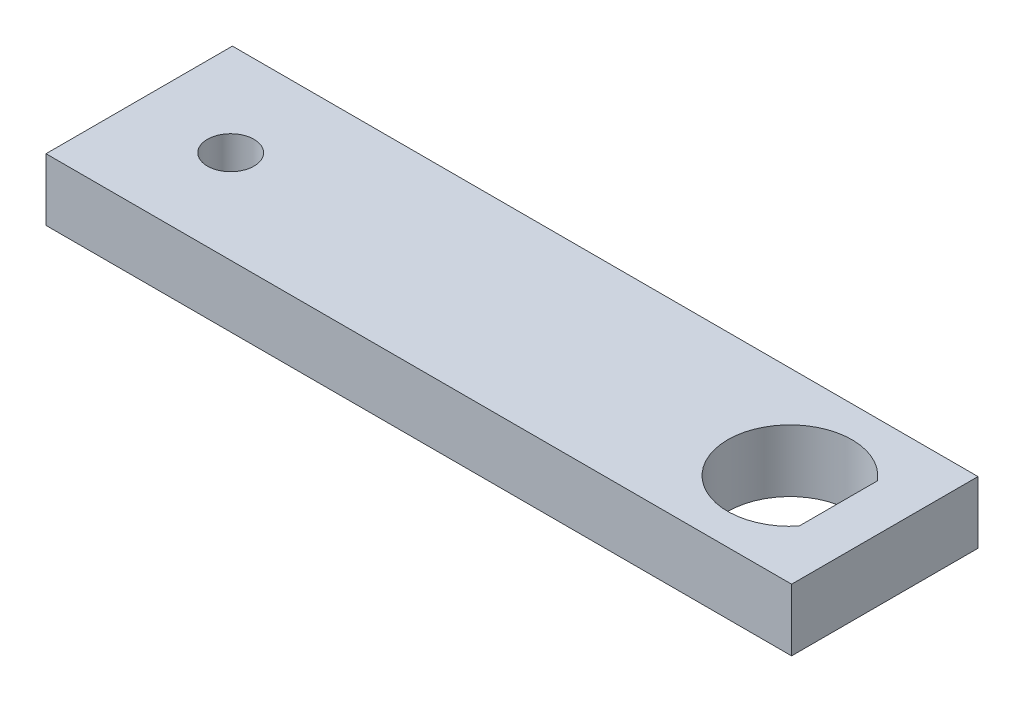
ISO-10303-21;
HEADER;
FILE_DESCRIPTION(('STEP AP214'),'2;1');
FILE_NAME('part.step','',(''),(''),'','','');
FILE_SCHEMA(('AUTOMOTIVE_DESIGN { 1 0 10303 214 1 1 1 1 }'));
ENDSEC;
DATA;
#1=APPLICATION_CONTEXT('core data for automotive mechanical design processes');
#2=APPLICATION_PROTOCOL_DEFINITION('international standard','automotive_design',2000,#1);
#3=PRODUCT_CONTEXT('',#1,'mechanical');
#4=PRODUCT('Part','Part','',(#3));
#5=PRODUCT_RELATED_PRODUCT_CATEGORY('part','',(#4));
#6=PRODUCT_DEFINITION_FORMATION('','',#4);
#7=PRODUCT_DEFINITION_CONTEXT('part definition',#1,'design');
#8=PRODUCT_DEFINITION('design','',#6,#7);
#9=PRODUCT_DEFINITION_SHAPE('','',#8);
#10=(LENGTH_UNIT() NAMED_UNIT(*) SI_UNIT(.MILLI.,.METRE.));
#11=(NAMED_UNIT(*) PLANE_ANGLE_UNIT() SI_UNIT($,.RADIAN.));
#12=(NAMED_UNIT(*) SI_UNIT($,.STERADIAN.) SOLID_ANGLE_UNIT());
#13=UNCERTAINTY_MEASURE_WITH_UNIT(LENGTH_MEASURE(1.E-05),#10,'distance_accuracy_value','');
#14=(GEOMETRIC_REPRESENTATION_CONTEXT(3) GLOBAL_UNCERTAINTY_ASSIGNED_CONTEXT((#13)) GLOBAL_UNIT_ASSIGNED_CONTEXT((#10,
#11,#12)) REPRESENTATION_CONTEXT('',''));
#15=CARTESIAN_POINT('',(0.,0.,0.));
#16=DIRECTION('',(0.,0.,1.));
#17=DIRECTION('',(1.,0.,0.));
#18=AXIS2_PLACEMENT_3D('',#15,#16,#17);
#19=CARTESIAN_POINT('',(0.,6.35,0.));
#20=DIRECTION('',(0.,1.,0.));
#21=DIRECTION('',(0.,0.,1.));
#22=AXIS2_PLACEMENT_3D('',#19,#20,#21);
#23=PLANE('',#22);
#24=CARTESIAN_POINT('',(28.4,6.35,0.));
#25=DIRECTION('',(0.,1.,0.));
#26=DIRECTION('',(0.,0.,1.));
#27=AXIS2_PLACEMENT_3D('',#24,#25,#26);
#28=CIRCLE('',#27,6.35);
#29=CARTESIAN_POINT('',(33.34,6.35,-3.98984962122634));
#30=VERTEX_POINT('',#29);
#31=CARTESIAN_POINT('',(33.34,6.35,3.98984962122634));
#32=VERTEX_POINT('',#31);
#33=EDGE_CURVE('E53',#30,#32,#28,.T.);
#34=ORIENTED_EDGE('',*,*,#33,.F.);
#35=DIRECTION('',(0.,0.,-1.));
#36=VECTOR('',#35,1.);
#37=CARTESIAN_POINT('',(33.34,6.35,3.98984962122634));
#38=LINE('',#37,#36);
#39=EDGE_CURVE('E103',#32,#30,#38,.T.);
#40=ORIENTED_EDGE('',*,*,#39,.F.);
#41=EDGE_LOOP('',(#34,#40));
#42=FACE_BOUND('',#41,.T.);
#43=DIRECTION('',(0.,0.,-1.));
#44=VECTOR('',#43,1.);
#45=CARTESIAN_POINT('',(38.1,6.35,-9.525));
#46=LINE('',#45,#44);
#47=CARTESIAN_POINT('',(38.1,6.35,9.525));
#48=VERTEX_POINT('',#47);
#49=CARTESIAN_POINT('',(38.1,6.35,-9.525));
#50=VERTEX_POINT('',#49);
#51=EDGE_CURVE('E116',#48,#50,#46,.T.);
#52=ORIENTED_EDGE('',*,*,#51,.T.);
#53=DIRECTION('',(-1.,0.,0.));
#54=VECTOR('',#53,1.);
#55=CARTESIAN_POINT('',(-38.1,6.35,-9.525));
#56=LINE('',#55,#54);
#57=CARTESIAN_POINT('',(-38.1,6.35,-9.525));
#58=VERTEX_POINT('',#57);
#59=EDGE_CURVE('E118',#50,#58,#56,.T.);
#60=ORIENTED_EDGE('',*,*,#59,.T.);
#61=DIRECTION('',(0.,0.,1.));
#62=VECTOR('',#61,1.);
#63=CARTESIAN_POINT('',(-38.1,6.35,-9.525));
#64=LINE('',#63,#62);
#65=CARTESIAN_POINT('',(-38.1,6.35,9.525));
#66=VERTEX_POINT('',#65);
#67=EDGE_CURVE('E125',#58,#66,#64,.T.);
#68=ORIENTED_EDGE('',*,*,#67,.T.);
#69=DIRECTION('',(1.,0.,0.));
#70=VECTOR('',#69,1.);
#71=CARTESIAN_POINT('',(-38.1,6.35,9.525));
#72=LINE('',#71,#70);
#73=EDGE_CURVE('E123',#66,#48,#72,.T.);
#74=ORIENTED_EDGE('',*,*,#73,.T.);
#75=EDGE_LOOP('',(#52,#60,#68,#74));
#76=FACE_BOUND('',#75,.T.);
#77=CARTESIAN_POINT('',(-28.75,6.35,0.));
#78=DIRECTION('',(0.,1.,0.));
#79=DIRECTION('',(0.,0.,1.));
#80=AXIS2_PLACEMENT_3D('',#77,#78,#79);
#81=CIRCLE('',#80,2.38);
#82=CARTESIAN_POINT('',(-28.75,6.35,2.38));
#83=VERTEX_POINT('',#82);
#84=EDGE_CURVE('E109',#83,#83,#81,.T.);
#85=ORIENTED_EDGE('',*,*,#84,.F.);
#86=EDGE_LOOP('',(#85));
#87=FACE_BOUND('',#86,.T.);
#88=ADVANCED_FACE('F39',(#42,#76,#87),#23,.T.);
#89=CARTESIAN_POINT('',(0.,0.,0.));
#90=DIRECTION('',(0.,1.,0.));
#91=DIRECTION('',(0.,0.,1.));
#92=AXIS2_PLACEMENT_3D('',#89,#90,#91);
#93=PLANE('',#92);
#94=DIRECTION('',(0.,0.,-1.));
#95=VECTOR('',#94,1.);
#96=CARTESIAN_POINT('',(33.34,0.,3.98984962122634));
#97=LINE('',#96,#95);
#98=CARTESIAN_POINT('',(33.34,0.,3.98984962122634));
#99=VERTEX_POINT('',#98);
#100=CARTESIAN_POINT('',(33.34,0.,-3.98984962122634));
#101=VERTEX_POINT('',#100);
#102=EDGE_CURVE('E92',#99,#101,#97,.T.);
#103=ORIENTED_EDGE('',*,*,#102,.T.);
#104=CARTESIAN_POINT('',(28.4,0.,0.));
#105=DIRECTION('',(0.,1.,0.));
#106=DIRECTION('',(0.,0.,1.));
#107=AXIS2_PLACEMENT_3D('',#104,#105,#106);
#108=CIRCLE('',#107,6.35);
#109=EDGE_CURVE('E56',#101,#99,#108,.T.);
#110=ORIENTED_EDGE('',*,*,#109,.T.);
#111=EDGE_LOOP('',(#103,#110));
#112=FACE_BOUND('',#111,.T.);
#113=DIRECTION('',(0.,0.,-1.));
#114=VECTOR('',#113,1.);
#115=CARTESIAN_POINT('',(38.1,0.,-9.525));
#116=LINE('',#115,#114);
#117=CARTESIAN_POINT('',(38.1,0.,9.525));
#118=VERTEX_POINT('',#117);
#119=CARTESIAN_POINT('',(38.1,0.,-9.525));
#120=VERTEX_POINT('',#119);
#121=EDGE_CURVE('E114',#118,#120,#116,.T.);
#122=ORIENTED_EDGE('',*,*,#121,.F.);
#123=DIRECTION('',(1.,0.,0.));
#124=VECTOR('',#123,1.);
#125=CARTESIAN_POINT('',(-38.1,0.,9.525));
#126=LINE('',#125,#124);
#127=CARTESIAN_POINT('',(-38.1,0.,9.525));
#128=VERTEX_POINT('',#127);
#129=EDGE_CURVE('E119',#128,#118,#126,.T.);
#130=ORIENTED_EDGE('',*,*,#129,.F.);
#131=DIRECTION('',(0.,0.,1.));
#132=VECTOR('',#131,1.);
#133=CARTESIAN_POINT('',(-38.1,0.,-9.525));
#134=LINE('',#133,#132);
#135=CARTESIAN_POINT('',(-38.1,0.,-9.525));
#136=VERTEX_POINT('',#135);
#137=EDGE_CURVE('E131',#136,#128,#134,.T.);
#138=ORIENTED_EDGE('',*,*,#137,.F.);
#139=DIRECTION('',(-1.,0.,0.));
#140=VECTOR('',#139,1.);
#141=CARTESIAN_POINT('',(-38.1,0.,-9.525));
#142=LINE('',#141,#140);
#143=EDGE_CURVE('E129',#120,#136,#142,.T.);
#144=ORIENTED_EDGE('',*,*,#143,.F.);
#145=EDGE_LOOP('',(#122,#130,#138,#144));
#146=FACE_BOUND('',#145,.T.);
#147=CARTESIAN_POINT('',(-28.75,0.,0.));
#148=DIRECTION('',(0.,1.,0.));
#149=DIRECTION('',(0.,0.,1.));
#150=AXIS2_PLACEMENT_3D('',#147,#148,#149);
#151=CIRCLE('',#150,2.38);
#152=CARTESIAN_POINT('',(-28.75,0.,2.38));
#153=VERTEX_POINT('',#152);
#154=EDGE_CURVE('E107',#153,#153,#151,.T.);
#155=ORIENTED_EDGE('',*,*,#154,.T.);
#156=EDGE_LOOP('',(#155));
#157=FACE_BOUND('',#156,.T.);
#158=ADVANCED_FACE('F101',(#112,#146,#157),#93,.F.);
#159=CARTESIAN_POINT('',(38.1,6.35,-9.525));
#160=DIRECTION('',(-1.,0.,0.));
#161=DIRECTION('',(0.,0.,1.));
#162=AXIS2_PLACEMENT_3D('',#159,#160,#161);
#163=PLANE('',#162);
#164=ORIENTED_EDGE('',*,*,#121,.T.);
#165=DIRECTION('',(0.,-1.,0.));
#166=VECTOR('',#165,1.);
#167=CARTESIAN_POINT('',(38.1,6.35,-9.525));
#168=LINE('',#167,#166);
#169=EDGE_CURVE('E11',#50,#120,#168,.T.);
#170=ORIENTED_EDGE('',*,*,#169,.F.);
#171=ORIENTED_EDGE('',*,*,#51,.F.);
#172=DIRECTION('',(0.,-1.,0.));
#173=VECTOR('',#172,1.);
#174=CARTESIAN_POINT('',(38.1,6.35,9.525));
#175=LINE('',#174,#173);
#176=EDGE_CURVE('E127',#48,#118,#175,.T.);
#177=ORIENTED_EDGE('',*,*,#176,.T.);
#178=EDGE_LOOP('',(#164,#170,#171,#177));
#179=FACE_BOUND('',#178,.T.);
#180=ADVANCED_FACE('F41',(#179),#163,.F.);
#181=CARTESIAN_POINT('',(-38.1,6.35,-9.525));
#182=DIRECTION('',(0.,0.,1.));
#183=DIRECTION('',(1.,0.,0.));
#184=AXIS2_PLACEMENT_3D('',#181,#182,#183);
#185=PLANE('',#184);
#186=ORIENTED_EDGE('',*,*,#143,.T.);
#187=DIRECTION('',(0.,-1.,0.));
#188=VECTOR('',#187,1.);
#189=CARTESIAN_POINT('',(-38.1,6.35,-9.525));
#190=LINE('',#189,#188);
#191=EDGE_CURVE('E50',#58,#136,#190,.T.);
#192=ORIENTED_EDGE('',*,*,#191,.F.);
#193=ORIENTED_EDGE('',*,*,#59,.F.);
#194=ORIENTED_EDGE('',*,*,#169,.T.);
#195=EDGE_LOOP('',(#186,#192,#193,#194));
#196=FACE_BOUND('',#195,.T.);
#197=ADVANCED_FACE('F158',(#196),#185,.F.);
#198=CARTESIAN_POINT('',(-38.1,6.35,-9.525));
#199=DIRECTION('',(1.,0.,0.));
#200=DIRECTION('',(0.,0.,-1.));
#201=AXIS2_PLACEMENT_3D('',#198,#199,#200);
#202=PLANE('',#201);
#203=ORIENTED_EDGE('',*,*,#137,.T.);
#204=DIRECTION('',(0.,-1.,0.));
#205=VECTOR('',#204,1.);
#206=CARTESIAN_POINT('',(-38.1,6.35,9.525));
#207=LINE('',#206,#205);
#208=EDGE_CURVE('E136',#66,#128,#207,.T.);
#209=ORIENTED_EDGE('',*,*,#208,.F.);
#210=ORIENTED_EDGE('',*,*,#67,.F.);
#211=ORIENTED_EDGE('',*,*,#191,.T.);
#212=EDGE_LOOP('',(#203,#209,#210,#211));
#213=FACE_BOUND('',#212,.T.);
#214=ADVANCED_FACE('F141',(#213),#202,.F.);
#215=CARTESIAN_POINT('',(-38.1,6.35,9.525));
#216=DIRECTION('',(0.,0.,-1.));
#217=DIRECTION('',(-1.,0.,0.));
#218=AXIS2_PLACEMENT_3D('',#215,#216,#217);
#219=PLANE('',#218);
#220=ORIENTED_EDGE('',*,*,#129,.T.);
#221=ORIENTED_EDGE('',*,*,#176,.F.);
#222=ORIENTED_EDGE('',*,*,#73,.F.);
#223=ORIENTED_EDGE('',*,*,#208,.T.);
#224=EDGE_LOOP('',(#220,#221,#222,#223));
#225=FACE_BOUND('',#224,.T.);
#226=ADVANCED_FACE('F151',(#225),#219,.F.);
#227=CARTESIAN_POINT('',(-28.75,6.35,0.));
#228=DIRECTION('',(0.,-1.,0.));
#229=DIRECTION('',(0.,0.,-1.));
#230=AXIS2_PLACEMENT_3D('',#227,#228,#229);
#231=CYLINDRICAL_SURFACE('',#230,2.38);
#232=ORIENTED_EDGE('',*,*,#84,.T.);
#233=EDGE_LOOP('',(#232));
#234=FACE_BOUND('',#233,.T.);
#235=ORIENTED_EDGE('',*,*,#154,.F.);
#236=EDGE_LOOP('',(#235));
#237=FACE_BOUND('',#236,.T.);
#238=ADVANCED_FACE('F173',(#234,#237),#231,.F.);
#239=CARTESIAN_POINT('',(28.4,0.,0.));
#240=DIRECTION('',(0.,1.,0.));
#241=DIRECTION('',(0.,0.,1.));
#242=AXIS2_PLACEMENT_3D('',#239,#240,#241);
#243=CYLINDRICAL_SURFACE('',#242,6.35);
#244=ORIENTED_EDGE('',*,*,#33,.T.);
#245=DIRECTION('',(0.,1.,0.));
#246=VECTOR('',#245,1.);
#247=CARTESIAN_POINT('',(33.34,0.,3.98984962122634));
#248=LINE('',#247,#246);
#249=EDGE_CURVE('E86',#99,#32,#248,.T.);
#250=ORIENTED_EDGE('',*,*,#249,.F.);
#251=ORIENTED_EDGE('',*,*,#109,.F.);
#252=DIRECTION('',(0.,1.,0.));
#253=VECTOR('',#252,1.);
#254=CARTESIAN_POINT('',(33.34,0.,-3.98984962122634));
#255=LINE('',#254,#253);
#256=EDGE_CURVE('E94',#101,#30,#255,.T.);
#257=ORIENTED_EDGE('',*,*,#256,.T.);
#258=EDGE_LOOP('',(#244,#250,#251,#257));
#259=FACE_BOUND('',#258,.T.);
#260=ADVANCED_FACE('F89',(#259),#243,.F.);
#261=CARTESIAN_POINT('',(33.34,0.,3.98984962122634));
#262=DIRECTION('',(1.,0.,0.));
#263=DIRECTION('',(0.,0.,-1.));
#264=AXIS2_PLACEMENT_3D('',#261,#262,#263);
#265=PLANE('',#264);
#266=ORIENTED_EDGE('',*,*,#39,.T.);
#267=ORIENTED_EDGE('',*,*,#256,.F.);
#268=ORIENTED_EDGE('',*,*,#102,.F.);
#269=ORIENTED_EDGE('',*,*,#249,.T.);
#270=EDGE_LOOP('',(#266,#267,#268,#269));
#271=FACE_BOUND('',#270,.T.);
#272=ADVANCED_FACE('F98',(#271),#265,.F.);
#273=CLOSED_SHELL('',(#88,#158,#180,#197,#214,#226,#238,#260,#272));
#274=MANIFOLD_SOLID_BREP('B2',#273);
#275=ADVANCED_BREP_SHAPE_REPRESENTATION('',(#18,#274),#14);
#276=SHAPE_DEFINITION_REPRESENTATION(#9,#275);
ENDSEC;
END-ISO-10303-21;
